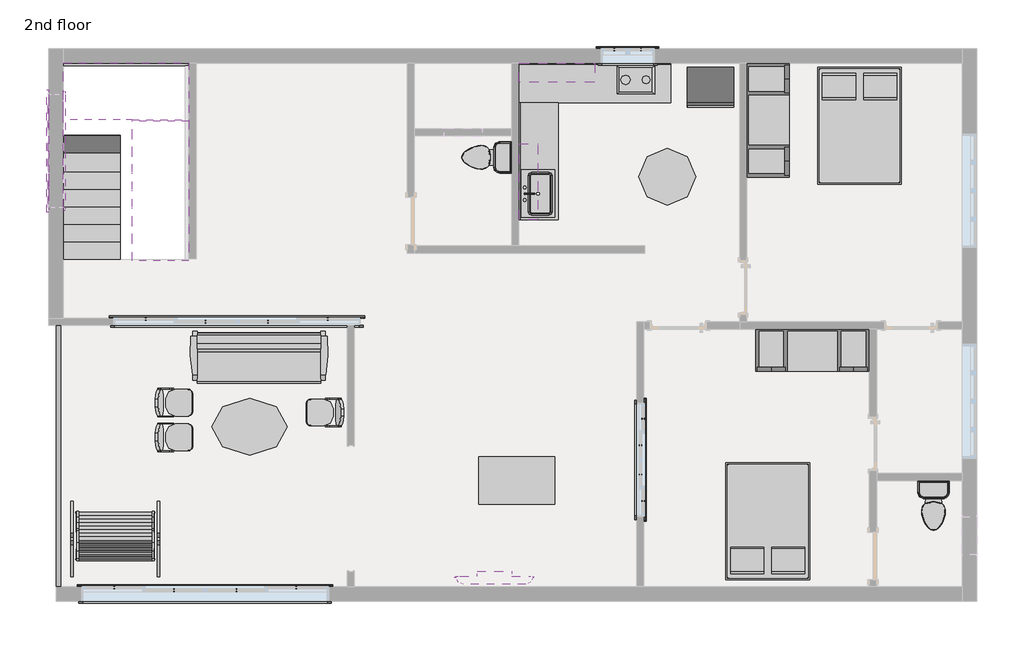
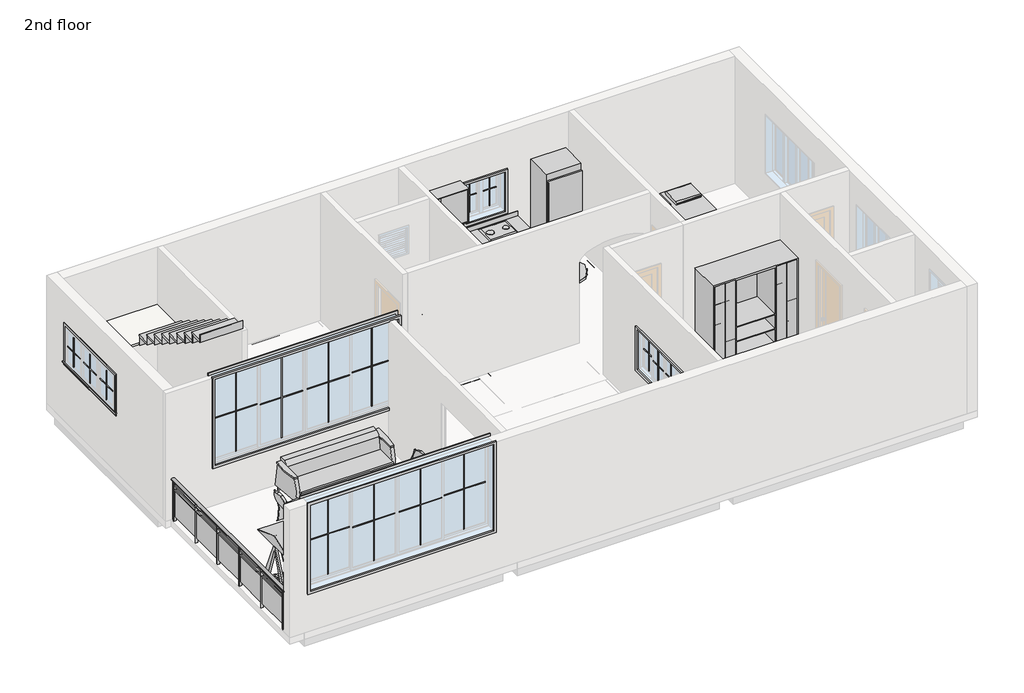
# One storey, part 2 of 2: 30 proxies, 21 furniture elements, 7 beams, 3 flow terminals, 2 stair flights, 1 railing, 1 slab.
# Revit data of these elements (continued)
# Elements 52, 53, 54 (IfcFurniture, "Seating-Auditorium : 18\" x 24\" x 30\"")
#   Phase Created = New Construction
#   Materials on its faces: "Steel, Paint Finish, Dark Gray, Matte", "Linen, Beige"
# Element 55 (IfcFurniture, "Sofa-Pensi : 84\"")
#   Phase Created = New Construction
#   Materials on its faces: "Cherry", "Linen, Beige", "Steel, Chrome Plated"
# Element 56 (IfcFurniture, "TV - Flat Screen : 50\"")
#   Stand = yes
#   Phase Created = New Construction
#   Materials on its faces: "TV - Black", "TV - Glass", "TV - Screen"
# Element 57 (IfcFurniture, "Table-Coffee Rectangular : 48\" x 30\"")
#   Phase Created = New Construction
#   Materials on its faces: "Metal - Chrome", "Glass - Clear, Grey"
# Element 58 (IfcFurniture, "Table-Dining Round w Chairs : 36\" Diameter")
#   Phase Created = New Construction
#   Materials on its faces: "Pine", "Laminate, Linen, Matte"
# Element 59 (IfcFurniture, "Table-Ellipse : 60\" x 48\"")
#   Phase Created = New Construction
#   Materials on its faces: "Birch"
# Elements 60, 61 (IfcFurniture, "Upper Cabinet-Pass-Thru w Glass : 48\" x 30\" x 12\"")
#   Phase Created = New Construction
#   Materials on its faces: "Glass", "Cabinet"
# Element 62 (IfcRailing, "Glass Panel - Bottom Fill")
#   Phase Created = New Construction
#   Materials on its faces: "Glass"
# Element 63 (IfcSlab, "Non-Monolithic Landing")
#   Phase Created = New Construction
# Elements 64, 65 (IfcStairFlight, "2\" Tread 1\" Nosing 1/4\" Riser")
#   Phase Created = New Construction
# Materials
#   "Concrete, Cast-in-Place gray": class "Concrete", colour RGB 192 192 192, transparency 0, Description = "Cast-in-place concrete", Cost = 0
#   "Metal - Chrome": class "Metal", colour RGB 247 247 247, transparency 0
#   "Metal - Steel, Polished": colour RGB 57 57 57, transparency 0
#   "Metal - Paint Finish - Ivory,Glossy": colour RGB 247 247 239, transparency 0
#   "Steel, Polished": class "Metal", colour RGB 57 57 57, transparency 0, Description = "Polished steel", Cost = 0
#   "Porcelain, Linen": class "Ceramic", colour RGB 249 239 230, transparency 0, Description = "Porcelain, linen", Cost = 0
#   "Laminate, Linen, Matte": class "Plastic", colour RGB 249 239 230, transparency 0, Description = "Plastic Laminate - Linen, Matte", Cost = 0
#   "Wood - Birch": class "Wood", colour RGB 224 178 126, transparency 0
#   "Laminate - Ivory, Matte": colour RGB 247 247 239, transparency 0
#   "Cabinets": colour RGB 249 249 249, transparency 0
#   "Cabinets - Handles": colour RGB 57 57 57, transparency 0
#   "Birch": class "Wood", colour RGB 224 178 126, transparency 0, Description = "Betula Alleghaniensis", Cost = 0
#   "Linen, White": class "Textile", colour RGB 247 247 239, transparency 0, Description = "Linen, white", Cost = 0
#   "Linen, Beige": class "Textile", colour RGB 249 239 230, transparency 0, Description = "Linen, beige", Cost = 0
#   "Steel, Paint Finish, Dark Gray, Matte": class "Metal", colour RGB 0 0 0, transparency 0, Description = "Steel, paint finish, dark gray, matte", Cost = 0
#   "Cherry": class "Wood", colour RGB 226 177 128, transparency 0, Description = "Prunus Serotina", Cost = 0
#   "Steel, Chrome Plated": class "Metal", colour RGB 17 17 17, transparency 0, Description = "Chromiuim plated steel", Cost = 0
#   "Glass - Clear, Grey": class "Glass", colour RGB 252 255 255, transparency 0.64
#   "Pine": class "Wood", colour RGB 223 192 134, transparency 0, Description = "Pinus Echinata", Cost = 0
#   "Clad - White": class "Wood", colour RGB 242 242 238, transparency 0, Cost = 0
#   "Wood - Stained": class "Wood", colour RGB 224 178 126, transparency 0, Cost = 0
#   "wood finish": class "Generic", colour RGB 120 120 120, transparency 0, Cost = 0
#   "steel": class "Generic", colour RGB 120 120 120, transparency 0, Cost = 0
#   "fabric": class "Generic", colour RGB 120 120 120, transparency 0, Cost = 0
#   "Cabinet": colour RGB 204 122 2, transparency 0
#   "Counter Top": class "Wood", colour RGB 226 177 128, transparency 0
#   "TV - Black": colour RGB 49 49 49, transparency 0
#   "TV - Glass": colour RGB 157 157 157, transparency 0.9
#   "TV - Screen": colour RGB 0 0 0, transparency 0
#   "Glass": class "Glass", colour RGB 0 128 192, transparency 0.75, Description = "Soda Lime Glass", Cost = 0
